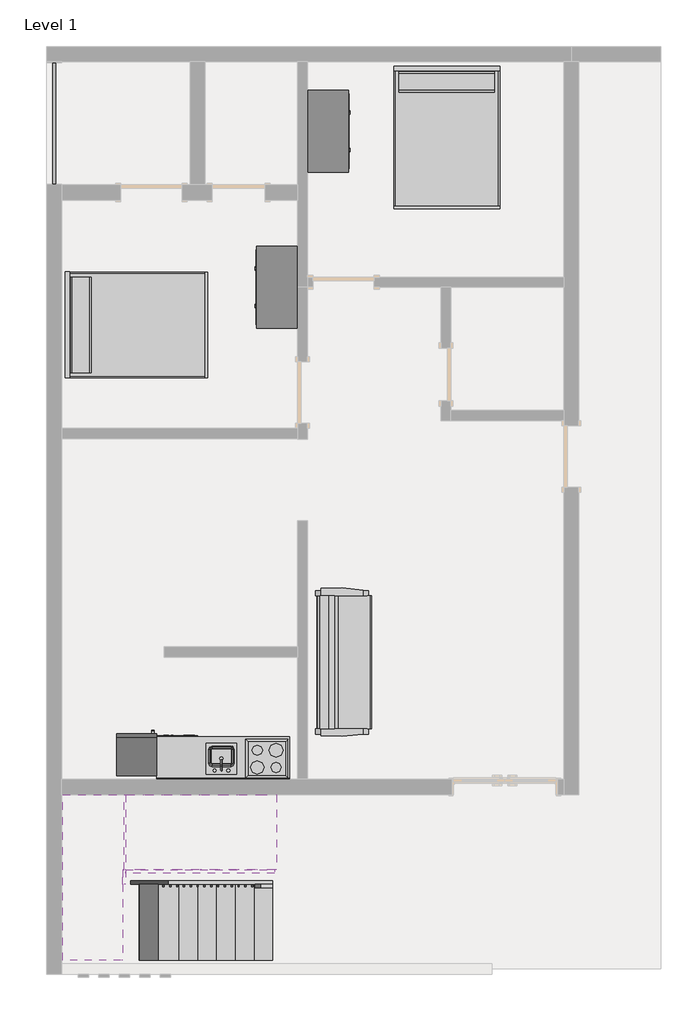
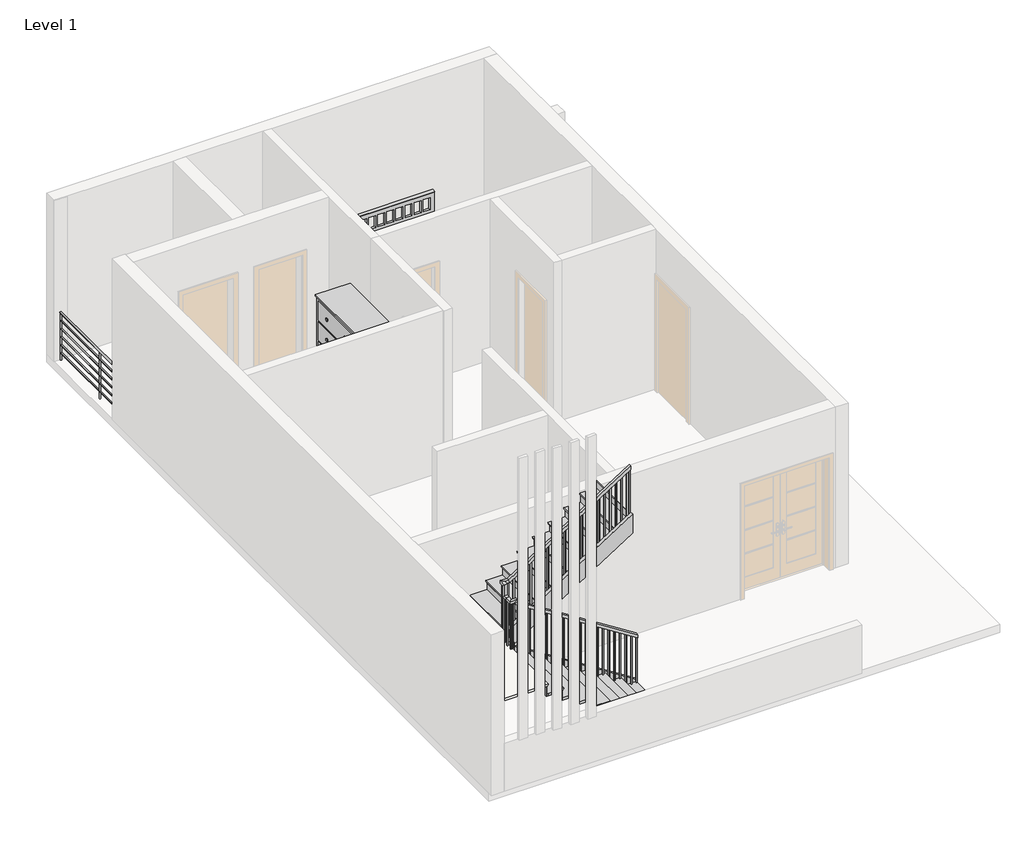
# One storey, part 2 of 2: 6 furniture elements, 4 proxies, 3 members, 2 railings, 2 stair flights, 1 flow terminal, 1 slab.
"""IFC4 building model written with IfcOpenShell, lengths in millimetres."""

from ifc_helpers import new_model, si_unit, point, frame, frame_2d, origin, origin_with_axes, place, context, project, spatial, polyline, circle_curve, trimmed, segment, composite_curve, outline, extrude, faceted_brep, transform, mapped, element, save
from components import proxy_a6faaae8, proxy_45b28599, kitchenette_medium_kitchenette_medium_844211aa, proxy_c523a7b7, flow_terminal_871c2e40, furniture_35c09872, furniture_c6510c7c, furniture_9fa109b2, furniture_aff9b2fb, non_monolithic_landing_c221236f, stair_flight_1352b5f3, stair_flight_ef2f52e6

model = new_model("IFC4")

# Units and contexts
model_context = context("Model", 3, world=origin())
ifc_project = project(units=[si_unit("LENGTHUNIT", "METRE", prefix="MILLI")], contexts=[model_context])

# Site, building, storey
site = spatial("IfcSite", under=ifc_project)
building = spatial("IfcBuilding", under=site)
storey = spatial("IfcBuildingStorey", under=building, Name="Level 1", Elevation=0.0)

# Proxies
placement = place(None, origin())
proxy_shape = proxy_a6faaae8(model_context)
element("IfcBuildingElementProxy", 1, Name="Cook Top-4 Unit2 : 22\" x 20\"", ObjectType="Cook Top-4 Unit2 : 22\" x 20\"", at=placement, inside=storey, context=model_context, shape_type="MappedRepresentation", body=[
    mapped(proxy_shape, transform((-8075.1683044, -841.1891189, 0.0), x_axis=(-1.0000000000000004, 0.0, 0.0), y_axis=(0.0, -1.0000000000000004, 0.0), z_axis=(0.0, 0.0, 1.0))),
])
proxy_2_shape = proxy_45b28599(model_context)
element("IfcBuildingElementProxy", 2, Name="Dishwasher : 24\" x 24\" x 34\"", ObjectType="Dishwasher : 24\" x 24\" x 34\"", at=placement, inside=storey, context=model_context, shape_type="MappedRepresentation", body=[
    mapped(proxy_2_shape, transform((-9026.3508359, -549.3395541, 0.0), x_axis=(-1.0000000000000004, 0.0, 0.0), y_axis=(0.0, -1.0000000000000004, 0.0), z_axis=(0.0, 0.0, 1.0))),
])
kitchenette_medium_kitchenette_medium_shape = kitchenette_medium_kitchenette_medium_844211aa(model_context)
element("IfcBuildingElementProxy", 3, Name="Kitchenette - Medium : Kitchenette - Medium", ObjectType="Kitchenette - Medium : Kitchenette - Medium", at=placement, inside=storey, context=model_context, shape_type="MappedRepresentation", body=[
    mapped(kitchenette_medium_kitchenette_medium_shape, transform((-8399.3305994, -1145.9891189, 0.0), x_axis=(-1.0000000000000004, 0.0, 0.0), y_axis=(0.0, -1.0000000000000004, 0.0), z_axis=(0.0, 0.0, 1.0))),
])
proxy_3_shape = proxy_c523a7b7(model_context)
element("IfcBuildingElementProxy", 4, Name="Refrigerator : 24\" x 25\" LH", ObjectType="Refrigerator : 24\" x 25\" LH", at=placement, inside=storey, context=model_context, shape_type="MappedRepresentation", body=[
    mapped(proxy_3_shape, transform((-10011.9183044, -795.5401474, 0.0), x_axis=(-1.0000000000000004, 0.0, 0.0), y_axis=(0.0, -1.0000000000000004, 0.0), z_axis=(0.0, 0.0, 1.0))),
])

# Flow terminal
flow_terminal_shape = flow_terminal_871c2e40(model_context)
element("IfcFlowTerminal", 5, ObjectType="Sink Kitchen-Island : 18\" x 18\"", at=placement, inside=storey, context=model_context, shape_type="MappedRepresentation", body=[
    mapped(flow_terminal_shape, transform((-8732.5790638, -838.8437178, -14.4), x_axis=(-1.0000000000000004, 0.0, 0.0), y_axis=(0.0, -1.0000000000000004, 0.0), z_axis=(0.0, 0.0, 1.0))),
])

# Furniture
furniture_shape = furniture_35c09872(model_context)
element("IfcFurniture", 6, ObjectType="Bed-Shaker : Queen 62\" x 83\"", at=placement, inside=storey, context=model_context, shape_type="MappedRepresentation", body=[
    mapped(furniture_shape, transform((-11059.6683044, 5629.4608811, 0.0), x_axis=(0.0, 1.0, 0.0), y_axis=(-1.0, 0.0, 0.0), z_axis=(0.0, 0.0, 1.0))),
])
element("IfcFurniture", 7, ObjectType="Bed-Shaker : Queen 62\" x 83\"", at=placement, inside=storey, context=model_context, shape_type="MappedRepresentation", body=[
    mapped(furniture_shape, transform((-5376.4183044, 9445.8108811, 0.0), x_axis=(1.0, 0.0, 0.0), y_axis=(0.0, 1.0, 0.0), z_axis=(0.0, 0.0, 1.0))),
])
furniture_2_shape = furniture_c6510c7c(model_context)
element("IfcFurniture", 8, ObjectType="Counter Top w Sink Hole : 24\" Depth", at=placement, inside=storey, context=model_context, shape_type="MappedRepresentation", body=[
    mapped(furniture_2_shape, transform((-8932.7305994, -1145.9891189, -14.4), x_axis=(-1.0000000000000004, 0.0, 0.0), y_axis=(0.0, -1.0000000000000004, 0.0), z_axis=(0.0, 0.0, 1.0))),
])
furniture_3_shape = furniture_9fa109b2(model_context)
element("IfcFurniture", 9, ObjectType="Dresser : 48\" x 72\" x 24\"", at=placement, inside=storey, context=model_context, shape_type="MappedRepresentation", body=[
    mapped(furniture_3_shape, transform((-7559.6053503, 5900.0176213, 0.0), x_axis=(0.0, -1.0000000000000004, 0.0), y_axis=(1.0000000000000004, 0.0, 0.0), z_axis=(0.0, 0.0, 1.0))),
])
element("IfcFurniture", 10, ObjectType="Dresser : 48\" x 72\" x 24\"", at=placement, inside=storey, context=model_context, shape_type="MappedRepresentation", body=[
    mapped(furniture_3_shape, transform((-7523.9312585, 8762.5041409, 0.0), x_axis=(0.0, 1.0000000000000009, 0.0), y_axis=(-1.0000000000000009, 0.0, 0.0), z_axis=(0.0, 0.0, 1.0))),
])
furniture_4_shape = furniture_aff9b2fb(model_context)
element("IfcFurniture", 11, ObjectType="Sofa-Pensi : 84\"", at=placement, inside=storey, context=model_context, shape_type="MappedRepresentation", body=[
    mapped(furniture_4_shape, transform((-6655.0584683, 315.3046311, 0.0), x_axis=(0.0, 1.0, 0.0), y_axis=(-1.0, 0.0, 0.0), z_axis=(0.0, 0.0, 1.0))),
])

# Members
element("IfcMember", 12, ObjectType="Stringer - 2\" Width", at=placement, inside=storey, context=model_context, shape_type="SweptSolid", body=[
    extrude(outline(polyline([(0.0, -7986.2683044), (215.0106437, -7986.2683044), (1605.083371, -10170.6683044), (1243.8010268, -10170.6683044), (0.0, -8216.1238337), (0.0, -7986.2683044)])), frame((0.0, -2706.1923176, 0.0), z_axis=(0.0, 1.0, 0.0), x_axis=(0.0, 0.0, 1.0)), (0.0, 0.0, 1.0), 50.8),
])
element("IfcMember", 13, ObjectType="Stringer - 2\" Width", at=placement, inside=storey, context=model_context, shape_type="SweptSolid", body=[
    extrude(outline(polyline([(1831.3742801, -10170.6683044), (1470.0919359, -10170.6683044), (2876.3282995, -7960.8683044), (3237.6106437, -7960.8683044), (1831.3742801, -10170.6683044)])), frame((0.0, -2542.9891189, 0.0), z_axis=(0.0, 1.0, 0.0), x_axis=(0.0, 0.0, 1.0)), (0.0, 0.0, 1.0), 50.8),
])
element("IfcMember", 14, ObjectType="Stringer - 2\" Width", at=placement, inside=storey, context=model_context, shape_type="SweptSolid", body=[
    extrude(outline(polyline([(-10170.6683044, -2706.1923176), (-10221.4683044, -2706.1923176), (-10221.4683044, -2492.1891189), (-10170.6683044, -2492.1891189), (-10170.6683044, -2706.1923176)])), frame((0.0, 0.0, 1371.6), z_axis=(0.0, 0.0, 1.0), x_axis=(1.0, 0.0, 0.0)), (0.0, 0.0, 1.0), 304.8),
])

# Railings
element("IfcRailing", 15, ObjectType="Handrail - Pipe", at=placement, inside=storey, context=model_context, shape_type="SweptSolid", body=[
    extrude(outline(composite_curve([segment(trimmed(circle_curve(frame_2d((895.35, -11237.4683044)), 19.05), [point((895.35, -11256.5183044))], [point((895.35, -11218.4183044))], False, "CARTESIAN"), True, "CONTINUOUS"), segment(trimmed(circle_curve(frame_2d((895.35, -11237.4683044)), 19.05), [point((895.35, -11218.4183044))], [point((895.35, -11256.5183044))], False, "CARTESIAN"), True, "CONTINUOUS")], self_intersect=False)), frame((0.0, 7705.9108811, 0.0), z_axis=(0.0, 1.0, 0.0), x_axis=(0.0, 0.0, 1.0)), (0.0, 0.0, 1.0), 1803.4),
    extrude(outline(composite_curve([segment(trimmed(circle_curve(frame_2d((749.3, -11237.4683044)), 12.7), [point((749.3, -11224.7683044))], [point((749.3, -11250.1683044))], False, "CARTESIAN"), True, "CONTINUOUS"), segment(trimmed(circle_curve(frame_2d((749.3, -11237.4683044)), 12.7), [point((749.3, -11250.1683044))], [point((749.3, -11224.7683044))], False, "CARTESIAN"), True, "CONTINUOUS")], self_intersect=False)), frame((0.0, 7705.9108811, 0.0), z_axis=(0.0, 1.0, 0.0), x_axis=(0.0, 0.0, 1.0)), (0.0, 0.0, 1.0), 1803.4),
    extrude(outline(composite_curve([segment(trimmed(circle_curve(frame_2d((596.9, -11237.4683044)), 12.7), [point((596.9, -11224.7683044))], [point((596.9, -11250.1683044))], False, "CARTESIAN"), True, "CONTINUOUS"), segment(trimmed(circle_curve(frame_2d((596.9, -11237.4683044)), 12.7), [point((596.9, -11250.1683044))], [point((596.9, -11224.7683044))], False, "CARTESIAN"), True, "CONTINUOUS")], self_intersect=False)), frame((0.0, 7705.9108811, 0.0), z_axis=(0.0, 1.0, 0.0), x_axis=(0.0, 0.0, 1.0)), (0.0, 0.0, 1.0), 1803.4),
    extrude(outline(composite_curve([segment(trimmed(circle_curve(frame_2d((444.5, -11237.4683044)), 12.7), [point((444.5, -11224.7683044))], [point((444.5, -11250.1683044))], False, "CARTESIAN"), True, "CONTINUOUS"), segment(trimmed(circle_curve(frame_2d((444.5, -11237.4683044)), 12.7), [point((444.5, -11250.1683044))], [point((444.5, -11224.7683044))], False, "CARTESIAN"), True, "CONTINUOUS")], self_intersect=False)), frame((0.0, 7705.9108811, 0.0), z_axis=(0.0, 1.0, 0.0), x_axis=(0.0, 0.0, 1.0)), (0.0, 0.0, 1.0), 1803.4),
    extrude(outline(composite_curve([segment(trimmed(circle_curve(frame_2d((292.1, -11237.4683044)), 12.7), [point((292.1, -11224.7683044))], [point((292.1, -11250.1683044))], False, "CARTESIAN"), True, "CONTINUOUS"), segment(trimmed(circle_curve(frame_2d((292.1, -11237.4683044)), 12.7), [point((292.1, -11250.1683044))], [point((292.1, -11224.7683044))], False, "CARTESIAN"), True, "CONTINUOUS")], self_intersect=False)), frame((0.0, 7705.9108811, 0.0), z_axis=(0.0, 1.0, 0.0), x_axis=(0.0, 0.0, 1.0)), (0.0, 0.0, 1.0), 1803.4),
    extrude(outline(composite_curve([segment(trimmed(circle_curve(frame_2d((139.7, -11237.4683044)), 12.7), [point((139.7, -11224.7683044))], [point((139.7, -11250.1683044))], False, "CARTESIAN"), True, "CONTINUOUS"), segment(trimmed(circle_curve(frame_2d((139.7, -11237.4683044)), 12.7), [point((139.7, -11250.1683044))], [point((139.7, -11224.7683044))], False, "CARTESIAN"), True, "CONTINUOUS")], self_intersect=False)), frame((0.0, 7705.9108811, 0.0), z_axis=(0.0, 1.0, 0.0), x_axis=(0.0, 0.0, 1.0)), (0.0, 0.0, 1.0), 1803.4),
    extrude(outline(composite_curve([segment(trimmed(circle_curve(frame_2d((-11237.4683044, 8290.1108811)), 12.7), [point((-11224.7683044, 8290.1108811))], [point((-11250.1683044, 8290.1108811))], False, "CARTESIAN"), True, "CONTINUOUS"), segment(trimmed(circle_curve(frame_2d((-11237.4683044, 8290.1108811)), 12.7), [point((-11250.1683044, 8290.1108811))], [point((-11224.7683044, 8290.1108811))], False, "CARTESIAN"), True, "CONTINUOUS")], self_intersect=False)), origin_with_axes(), (0.0, 0.0, 1.0), 876.3),
    extrude(outline(composite_curve([segment(trimmed(circle_curve(frame_2d((-11237.4683044, 7718.6108811)), 12.7), [point((-11224.7683044, 7718.6108811))], [point((-11250.1683044, 7718.6108811))], False, "CARTESIAN"), True, "CONTINUOUS"), segment(trimmed(circle_curve(frame_2d((-11237.4683044, 7718.6108811)), 12.7), [point((-11250.1683044, 7718.6108811))], [point((-11224.7683044, 7718.6108811))], False, "CARTESIAN"), True, "CONTINUOUS")], self_intersect=False)), origin_with_axes(), (0.0, 0.0, 1.0), 876.3),
    extrude(outline(composite_curve([segment(trimmed(circle_curve(frame_2d((-11237.4683044, 9496.6108811)), 12.7), [point((-11224.7683044, 9496.6108811))], [point((-11250.1683044, 9496.6108811))], False, "CARTESIAN"), True, "CONTINUOUS"), segment(trimmed(circle_curve(frame_2d((-11237.4683044, 9496.6108811)), 12.7), [point((-11250.1683044, 9496.6108811))], [point((-11224.7683044, 9496.6108811))], False, "CARTESIAN"), True, "CONTINUOUS")], self_intersect=False)), origin_with_axes(), (0.0, 0.0, 1.0), 876.3),
])
element("IfcRailing", 16, ObjectType="Handrail - Rectangular", at=placement, inside=storey, context=model_context, shape_type="SolidModel", body=[
    faceted_brep([(-7986.2683044, -2756.9923176, 1092.2), (-7986.2683044, -2756.9923176, 1031.986276), (-7986.2683044, -2706.1923176, 1031.986276), (-7986.2683044, -2706.1923176, 1092.2), (-10145.2683044, -2756.9923176, 2466.1090909), (-10196.0683044, -2756.9923176, 2438.2226396), (-10196.0683044, -2706.1923176, 2438.2226396), (-10145.2683044, -2706.1923176, 2466.1090909), (-10145.2683044, -2756.9923176, 2514.6), (-10196.0683044, -2756.9923176, 2463.8), (-10196.0683044, -2706.1923176, 2463.8), (-10145.2683044, -2706.1923176, 2514.6), (-10272.2683044, -2756.9923176, 2514.6), (-10272.2683044, -2756.9923176, 2463.8), (-10221.4683044, -2706.1923176, 2463.8), (-10221.4683044, -2706.1923176, 2514.6), (-10272.2683044, -2629.9923176, 2514.6), (-10272.2683044, -2629.9923176, 2463.8), (-10221.4683044, -2629.9923176, 2463.8), (-10221.4683044, -2629.9923176, 2514.6), (-10272.2683044, -2568.3891189, 2514.6), (-10272.2683044, -2517.5891189, 2463.8), (-10221.4683044, -2517.5891189, 2463.8), (-10221.4683044, -2568.3891189, 2514.6), (-10272.2683044, -2568.3891189, 2724.7272727), (-10272.2683044, -2517.5891189, 2673.9272727), (-10221.4683044, -2517.5891189, 2673.9272727), (-10221.4683044, -2568.3891189, 2724.7272727), (-7960.8683044, -2441.3891189, 4114.8), (-7960.8683044, -2492.1891189, 4114.8), (-7960.8683044, -2492.1891189, 4054.586276), (-7960.8683044, -2441.3891189, 4054.586276), (-10130.4753095, -2441.3891189, 2673.9272727), (-10145.2683044, -2441.3891189, 2724.7272727), (-10130.4753095, -2492.1891189, 2673.9272727), (-10145.2683044, -2492.1891189, 2724.7272727), (-10272.2683044, -2441.3891189, 2724.7272727), (-10272.2683044, -2441.3891189, 2673.9272727), (-10221.4683044, -2492.1891189, 2673.9272727), (-10221.4683044, -2492.1891189, 2724.7272727)], [[[0, 1, 2, 3]], [[1, 0, 4, 5]], [[2, 1, 5, 6]], [[3, 2, 6, 7]], [[0, 3, 7, 4]], [[5, 4, 8, 9]], [[6, 5, 9, 10]], [[7, 6, 10, 11]], [[4, 7, 11, 8]], [[9, 8, 12, 13]], [[10, 9, 13, 14]], [[11, 10, 14, 15]], [[8, 11, 15, 12]], [[13, 12, 16, 17]], [[14, 13, 17, 18]], [[15, 14, 18, 19]], [[12, 15, 19, 16]], [[17, 16, 20, 21]], [[18, 17, 21, 22]], [[19, 18, 22, 23]], [[16, 19, 23, 20]], [[21, 20, 24, 25]], [[22, 21, 25, 26]], [[23, 22, 26, 27]], [[20, 23, 27, 24]], [[28, 29, 30, 31]], [[32, 33, 28, 31]], [[34, 32, 31, 30]], [[35, 34, 30, 29]], [[33, 35, 29, 28]], [[25, 24, 36, 37]], [[26, 25, 37, 38]], [[27, 26, 38, 39]], [[24, 27, 39, 36]], [[37, 36, 33, 32]], [[38, 37, 32, 34]], [[39, 38, 34, 35]], [[36, 39, 35, 33]]]),
    extrude(outline(polyline([(4028.3203669, -8002.1433044), (4016.1976396, -8021.1933044), (3022.6, -8021.1933044), (3022.6, -8002.1433044), (4028.3203669, -8002.1433044)])), frame((0.0, -2476.3141189, 0.0), z_axis=(0.0, 1.0, 0.0), x_axis=(0.0, 0.0, 1.0)), (0.0, 0.0, 1.0), 19.05),
    extrude(outline(polyline([(3963.6658214, -8103.7433044), (3951.5430941, -8122.7933044), (3022.6, -8122.7933044), (3022.6, -8103.7433044), (3963.6658214, -8103.7433044)])), frame((0.0, -2476.3141189, 0.0), z_axis=(0.0, 1.0, 0.0), x_axis=(0.0, 0.0, 1.0)), (0.0, 0.0, 1.0), 19.05),
    extrude(outline(polyline([(3899.011276, -8205.3433044), (3886.8885487, -8224.3933044), (3022.6, -8224.3933044), (3022.6, -8205.3433044), (3899.011276, -8205.3433044)])), frame((0.0, -2476.3141189, 0.0), z_axis=(0.0, 1.0, 0.0), x_axis=(0.0, 0.0, 1.0)), (0.0, 0.0, 1.0), 19.05),
    extrude(outline(polyline([(3834.3567305, -8306.9433044), (3822.2340032, -8325.9933044), (2844.8, -8325.9933044), (2844.8, -8306.9433044), (3834.3567305, -8306.9433044)])), frame((0.0, -2476.3141189, 0.0), z_axis=(0.0, 1.0, 0.0), x_axis=(0.0, 0.0, 1.0)), (0.0, 0.0, 1.0), 19.05),
    extrude(outline(polyline([(3769.7021851, -8408.5433044), (3757.5794578, -8427.5933044), (2844.8, -8427.5933044), (2844.8, -8408.5433044), (3769.7021851, -8408.5433044)])), frame((0.0, -2476.3141189, 0.0), z_axis=(0.0, 1.0, 0.0), x_axis=(0.0, 0.0, 1.0)), (0.0, 0.0, 1.0), 19.05),
    extrude(outline(polyline([(3705.0476396, -8510.1433044), (3692.9249123, -8529.1933044), (2844.8, -8529.1933044), (2844.8, -8510.1433044), (3705.0476396, -8510.1433044)])), frame((0.0, -2476.3141189, 0.0), z_axis=(0.0, 1.0, 0.0), x_axis=(0.0, 0.0, 1.0)), (0.0, 0.0, 1.0), 19.05),
    extrude(outline(polyline([(3640.3930941, -8611.7433044), (3628.2703669, -8630.7933044), (2667.0, -8630.7933044), (2667.0, -8611.7433044), (3640.3930941, -8611.7433044)])), frame((0.0, -2476.3141189, 0.0), z_axis=(0.0, 1.0, 0.0), x_axis=(0.0, 0.0, 1.0)), (0.0, 0.0, 1.0), 19.05),
    extrude(outline(polyline([(3575.7385487, -8713.3433044), (3563.6158214, -8732.3933044), (2667.0, -8732.3933044), (2667.0, -8713.3433044), (3575.7385487, -8713.3433044)])), frame((0.0, -2476.3141189, 0.0), z_axis=(0.0, 1.0, 0.0), x_axis=(0.0, 0.0, 1.0)), (0.0, 0.0, 1.0), 19.05),
    extrude(outline(polyline([(3511.0840032, -8814.9433044), (3498.961276, -8833.9933044), (2489.2, -8833.9933044), (2489.2, -8814.9433044), (3511.0840032, -8814.9433044)])), frame((0.0, -2476.3141189, 0.0), z_axis=(0.0, 1.0, 0.0), x_axis=(0.0, 0.0, 1.0)), (0.0, 0.0, 1.0), 19.05),
    extrude(outline(polyline([(3446.4294578, -8916.5433044), (3434.3067305, -8935.5933044), (2489.2, -8935.5933044), (2489.2, -8916.5433044), (3446.4294578, -8916.5433044)])), frame((0.0, -2476.3141189, 0.0), z_axis=(0.0, 1.0, 0.0), x_axis=(0.0, 0.0, 1.0)), (0.0, 0.0, 1.0), 19.05),
    extrude(outline(polyline([(3381.7749123, -9018.1433044), (3369.6521851, -9037.1933044), (2489.2, -9037.1933044), (2489.2, -9018.1433044), (3381.7749123, -9018.1433044)])), frame((0.0, -2476.3141189, 0.0), z_axis=(0.0, 1.0, 0.0), x_axis=(0.0, 0.0, 1.0)), (0.0, 0.0, 1.0), 19.05),
    extrude(outline(polyline([(3317.1203669, -9119.7433044), (3304.9976396, -9138.7933044), (2311.4, -9138.7933044), (2311.4, -9119.7433044), (3317.1203669, -9119.7433044)])), frame((0.0, -2476.3141189, 0.0), z_axis=(0.0, 1.0, 0.0), x_axis=(0.0, 0.0, 1.0)), (0.0, 0.0, 1.0), 19.05),
    extrude(outline(polyline([(3252.4658214, -9221.3433044), (3240.3430941, -9240.3933044), (2311.4, -9240.3933044), (2311.4, -9221.3433044), (3252.4658214, -9221.3433044)])), frame((0.0, -2476.3141189, 0.0), z_axis=(0.0, 1.0, 0.0), x_axis=(0.0, 0.0, 1.0)), (0.0, 0.0, 1.0), 19.05),
    extrude(outline(polyline([(3187.811276, -9322.9433044), (3175.6885487, -9341.9933044), (2311.4, -9341.9933044), (2311.4, -9322.9433044), (3187.811276, -9322.9433044)])), frame((0.0, -2476.3141189, 0.0), z_axis=(0.0, 1.0, 0.0), x_axis=(0.0, 0.0, 1.0)), (0.0, 0.0, 1.0), 19.05),
    extrude(outline(polyline([(3123.1567305, -9424.5433044), (3111.0340032, -9443.5933044), (2133.6, -9443.5933044), (2133.6, -9424.5433044), (3123.1567305, -9424.5433044)])), frame((0.0, -2476.3141189, 0.0), z_axis=(0.0, 1.0, 0.0), x_axis=(0.0, 0.0, 1.0)), (0.0, 0.0, 1.0), 19.05),
    extrude(outline(polyline([(3058.5021851, -9526.1433044), (3046.3794578, -9545.1933044), (2133.6, -9545.1933044), (2133.6, -9526.1433044), (3058.5021851, -9526.1433044)])), frame((0.0, -2476.3141189, 0.0), z_axis=(0.0, 1.0, 0.0), x_axis=(0.0, 0.0, 1.0)), (0.0, 0.0, 1.0), 19.05),
    extrude(outline(polyline([(2993.8476396, -9627.7433044), (2981.7249123, -9646.7933044), (2133.6, -9646.7933044), (2133.6, -9627.7433044), (2993.8476396, -9627.7433044)])), frame((0.0, -2476.3141189, 0.0), z_axis=(0.0, 1.0, 0.0), x_axis=(0.0, 0.0, 1.0)), (0.0, 0.0, 1.0), 19.05),
    extrude(outline(polyline([(2929.1930941, -9729.3433044), (2917.0703669, -9748.3933044), (1955.8, -9748.3933044), (1955.8, -9729.3433044), (2929.1930941, -9729.3433044)])), frame((0.0, -2476.3141189, 0.0), z_axis=(0.0, 1.0, 0.0), x_axis=(0.0, 0.0, 1.0)), (0.0, 0.0, 1.0), 19.05),
    extrude(outline(polyline([(2864.5385487, -9830.9433044), (2852.4158214, -9849.9933044), (1955.8, -9849.9933044), (1955.8, -9830.9433044), (2864.5385487, -9830.9433044)])), frame((0.0, -2476.3141189, 0.0), z_axis=(0.0, 1.0, 0.0), x_axis=(0.0, 0.0, 1.0)), (0.0, 0.0, 1.0), 19.05),
    extrude(outline(polyline([(2799.8840032, -9932.5433044), (2787.761276, -9951.5933044), (1778.0, -9951.5933044), (1778.0, -9932.5433044), (2799.8840032, -9932.5433044)])), frame((0.0, -2476.3141189, 0.0), z_axis=(0.0, 1.0, 0.0), x_axis=(0.0, 0.0, 1.0)), (0.0, 0.0, 1.0), 19.05),
    extrude(outline(polyline([(2735.2294578, -10034.1433044), (2723.1067305, -10053.1933044), (1778.0, -10053.1933044), (1778.0, -10034.1433044), (2735.2294578, -10034.1433044)])), frame((0.0, -2476.3141189, 0.0), z_axis=(0.0, 1.0, 0.0), x_axis=(0.0, 0.0, 1.0)), (0.0, 0.0, 1.0), 19.05),
    extrude(outline(polyline([(-10154.7933044, -2476.3141189), (-10154.7933044, -2457.2641189), (-10135.7433044, -2457.2641189), (-10135.7433044, -2476.3141189), (-10154.7933044, -2476.3141189)])), frame((0.0, 0.0, 1778.0), z_axis=(0.0, 0.0, 1.0), x_axis=(1.0, 0.0, 0.0)), (0.0, 0.0, 1.0), 895.9272727),
    extrude(outline(polyline([(-10237.3433044, -2537.9173176), (-10256.3933044, -2537.9173176), (-10256.3933044, -2518.8673176), (-10237.3433044, -2518.8673176), (-10237.3433044, -2537.9173176)])), frame((0.0, 0.0, 1600.2), z_axis=(0.0, 0.0, 1.0), x_axis=(1.0, 0.0, 0.0)), (0.0, 0.0, 1.0), 863.6),
    extrude(outline(polyline([(-10237.3433044, -2639.5173176), (-10256.3933044, -2639.5173176), (-10256.3933044, -2620.4673176), (-10237.3433044, -2620.4673176), (-10237.3433044, -2639.5173176)])), frame((0.0, 0.0, 1600.2), z_axis=(0.0, 0.0, 1.0), x_axis=(1.0, 0.0, 0.0)), (0.0, 0.0, 1.0), 863.6),
    extrude(outline(polyline([(2383.6703669, -10110.3433044), (2395.7930941, -10129.3933044), (1422.4, -10129.3933044), (1422.4, -10110.3433044), (2383.6703669, -10110.3433044)])), frame((0.0, -2741.1173176, 0.0), z_axis=(0.0, 1.0, 0.0), x_axis=(0.0, 0.0, 1.0)), (0.0, 0.0, 1.0), 19.05),
    extrude(outline(polyline([(2319.0158214, -10008.7433044), (2331.1385487, -10027.7933044), (1422.4, -10027.7933044), (1422.4, -10008.7433044), (2319.0158214, -10008.7433044)])), frame((0.0, -2741.1173176, 0.0), z_axis=(0.0, 1.0, 0.0), x_axis=(0.0, 0.0, 1.0)), (0.0, 0.0, 1.0), 19.05),
    extrude(outline(polyline([(2254.361276, -9907.1433044), (2266.4840032, -9926.1933044), (1244.6, -9926.1933044), (1244.6, -9907.1433044), (2254.361276, -9907.1433044)])), frame((0.0, -2741.1173176, 0.0), z_axis=(0.0, 1.0, 0.0), x_axis=(0.0, 0.0, 1.0)), (0.0, 0.0, 1.0), 19.05),
    extrude(outline(polyline([(2189.7067305, -9805.5433044), (2201.8294578, -9824.5933044), (1244.6, -9824.5933044), (1244.6, -9805.5433044), (2189.7067305, -9805.5433044)])), frame((0.0, -2741.1173176, 0.0), z_axis=(0.0, 1.0, 0.0), x_axis=(0.0, 0.0, 1.0)), (0.0, 0.0, 1.0), 19.05),
    extrude(outline(polyline([(2125.0521851, -9703.9433044), (2137.1749123, -9722.9933044), (1244.6, -9722.9933044), (1244.6, -9703.9433044), (2125.0521851, -9703.9433044)])), frame((0.0, -2741.1173176, 0.0), z_axis=(0.0, 1.0, 0.0), x_axis=(0.0, 0.0, 1.0)), (0.0, 0.0, 1.0), 19.05),
    extrude(outline(polyline([(2060.3976396, -9602.3433044), (2072.5203669, -9621.3933044), (1066.8, -9621.3933044), (1066.8, -9602.3433044), (2060.3976396, -9602.3433044)])), frame((0.0, -2741.1173176, 0.0), z_axis=(0.0, 1.0, 0.0), x_axis=(0.0, 0.0, 1.0)), (0.0, 0.0, 1.0), 19.05),
    extrude(outline(polyline([(1995.7430941, -9500.7433044), (2007.8658214, -9519.7933044), (1066.8, -9519.7933044), (1066.8, -9500.7433044), (1995.7430941, -9500.7433044)])), frame((0.0, -2741.1173176, 0.0), z_axis=(0.0, 1.0, 0.0), x_axis=(0.0, 0.0, 1.0)), (0.0, 0.0, 1.0), 19.05),
    extrude(outline(polyline([(1931.0885487, -9399.1433044), (1943.211276, -9418.1933044), (1066.8, -9418.1933044), (1066.8, -9399.1433044), (1931.0885487, -9399.1433044)])), frame((0.0, -2741.1173176, 0.0), z_axis=(0.0, 1.0, 0.0), x_axis=(0.0, 0.0, 1.0)), (0.0, 0.0, 1.0), 19.05),
    extrude(outline(polyline([(1866.4340032, -9297.5433044), (1878.5567305, -9316.5933044), (889.0, -9316.5933044), (889.0, -9297.5433044), (1866.4340032, -9297.5433044)])), frame((0.0, -2741.1173176, 0.0), z_axis=(0.0, 1.0, 0.0), x_axis=(0.0, 0.0, 1.0)), (0.0, 0.0, 1.0), 19.05),
    extrude(outline(polyline([(1801.7794578, -9195.9433044), (1813.9021851, -9214.9933044), (889.0, -9214.9933044), (889.0, -9195.9433044), (1801.7794578, -9195.9433044)])), frame((0.0, -2741.1173176, 0.0), z_axis=(0.0, 1.0, 0.0), x_axis=(0.0, 0.0, 1.0)), (0.0, 0.0, 1.0), 19.05),
    extrude(outline(polyline([(1737.1249123, -9094.3433044), (1749.2476396, -9113.3933044), (889.0, -9113.3933044), (889.0, -9094.3433044), (1737.1249123, -9094.3433044)])), frame((0.0, -2741.1173176, 0.0), z_axis=(0.0, 1.0, 0.0), x_axis=(0.0, 0.0, 1.0)), (0.0, 0.0, 1.0), 19.05),
    extrude(outline(polyline([(1672.4703669, -8992.7433044), (1684.5930941, -9011.7933044), (711.2, -9011.7933044), (711.2, -8992.7433044), (1672.4703669, -8992.7433044)])), frame((0.0, -2741.1173176, 0.0), z_axis=(0.0, 1.0, 0.0), x_axis=(0.0, 0.0, 1.0)), (0.0, 0.0, 1.0), 19.05),
    extrude(outline(polyline([(1607.8158214, -8891.1433044), (1619.9385487, -8910.1933044), (711.2, -8910.1933044), (711.2, -8891.1433044), (1607.8158214, -8891.1433044)])), frame((0.0, -2741.1173176, 0.0), z_axis=(0.0, 1.0, 0.0), x_axis=(0.0, 0.0, 1.0)), (0.0, 0.0, 1.0), 19.05),
    extrude(outline(polyline([(1543.161276, -8789.5433044), (1555.2840032, -8808.5933044), (533.4, -8808.5933044), (533.4, -8789.5433044), (1543.161276, -8789.5433044)])), frame((0.0, -2741.1173176, 0.0), z_axis=(0.0, 1.0, 0.0), x_axis=(0.0, 0.0, 1.0)), (0.0, 0.0, 1.0), 19.05),
    extrude(outline(polyline([(1478.5067305, -8687.9433044), (1490.6294578, -8706.9933044), (533.4, -8706.9933044), (533.4, -8687.9433044), (1478.5067305, -8687.9433044)])), frame((0.0, -2741.1173176, 0.0), z_axis=(0.0, 1.0, 0.0), x_axis=(0.0, 0.0, 1.0)), (0.0, 0.0, 1.0), 19.05),
    extrude(outline(polyline([(1413.8521851, -8586.3433044), (1425.9749123, -8605.3933044), (533.4, -8605.3933044), (533.4, -8586.3433044), (1413.8521851, -8586.3433044)])), frame((0.0, -2741.1173176, 0.0), z_axis=(0.0, 1.0, 0.0), x_axis=(0.0, 0.0, 1.0)), (0.0, 0.0, 1.0), 19.05),
    extrude(outline(polyline([(1349.1976396, -8484.7433044), (1361.3203669, -8503.7933044), (355.6, -8503.7933044), (355.6, -8484.7433044), (1349.1976396, -8484.7433044)])), frame((0.0, -2741.1173176, 0.0), z_axis=(0.0, 1.0, 0.0), x_axis=(0.0, 0.0, 1.0)), (0.0, 0.0, 1.0), 19.05),
    extrude(outline(polyline([(1284.5430941, -8383.1433044), (1296.6658214, -8402.1933044), (355.6, -8402.1933044), (355.6, -8383.1433044), (1284.5430941, -8383.1433044)])), frame((0.0, -2741.1173176, 0.0), z_axis=(0.0, 1.0, 0.0), x_axis=(0.0, 0.0, 1.0)), (0.0, 0.0, 1.0), 19.05),
    extrude(outline(polyline([(1219.8885487, -8281.5433044), (1232.011276, -8300.5933044), (355.6, -8300.5933044), (355.6, -8281.5433044), (1219.8885487, -8281.5433044)])), frame((0.0, -2741.1173176, 0.0), z_axis=(0.0, 1.0, 0.0), x_axis=(0.0, 0.0, 1.0)), (0.0, 0.0, 1.0), 19.05),
    extrude(outline(polyline([(1155.2340032, -8179.9433044), (1167.3567305, -8198.9933044), (177.8, -8198.9933044), (177.8, -8179.9433044), (1155.2340032, -8179.9433044)])), frame((0.0, -2741.1173176, 0.0), z_axis=(0.0, 1.0, 0.0), x_axis=(0.0, 0.0, 1.0)), (0.0, 0.0, 1.0), 19.05),
    extrude(outline(polyline([(1090.5794578, -8078.3433044), (1102.7021851, -8097.3933044), (177.8, -8097.3933044), (177.8, -8078.3433044), (1090.5794578, -8078.3433044)])), frame((0.0, -2741.1173176, 0.0), z_axis=(0.0, 1.0, 0.0), x_axis=(0.0, 0.0, 1.0)), (0.0, 0.0, 1.0), 19.05),
    extrude(outline(polyline([(-10256.3933044, -2476.3141189), (-10256.3933044, -2457.2641189), (-10237.3433044, -2457.2641189), (-10237.3433044, -2476.3141189), (-10256.3933044, -2476.3141189)])), frame((0.0, 0.0, 1600.2), z_axis=(0.0, 0.0, 1.0), x_axis=(1.0, 0.0, 0.0)), (0.0, 0.0, 1.0), 1073.7272727),
    extrude(outline(polyline([(-10237.3433044, -2722.0673176), (-10237.3433044, -2741.1173176), (-10256.3933044, -2741.1173176), (-10256.3933044, -2722.0673176), (-10237.3433044, -2722.0673176)])), frame((0.0, 0.0, 1600.2), z_axis=(0.0, 0.0, 1.0), x_axis=(1.0, 0.0, 0.0)), (0.0, 0.0, 1.0), 863.6),
    extrude(outline(polyline([(-10211.9433044, -2722.0673176), (-10211.9433044, -2741.1173176), (-10230.9933044, -2741.1173176), (-10230.9933044, -2722.0673176), (-10211.9433044, -2722.0673176)])), frame((0.0, 0.0, 1600.2), z_axis=(0.0, 0.0, 1.0), x_axis=(1.0, 0.0, 0.0)), (0.0, 0.0, 1.0), 863.6),
    extrude(outline(polyline([(4054.586276, -7960.8683044), (4042.4635487, -7979.9183044), (3022.6, -7979.9183044), (3022.6, -7960.8683044), (4054.586276, -7960.8683044)])), frame((0.0, -2476.3141189, 0.0), z_axis=(0.0, 1.0, 0.0), x_axis=(0.0, 0.0, 1.0)), (0.0, 0.0, 1.0), 19.05),
    extrude(outline(polyline([(1031.986276, -7986.2683044), (1044.1090032, -8005.3183044), (177.8, -8005.3183044), (177.8, -7986.2683044), (1031.986276, -7986.2683044)])), frame((0.0, -2741.1173176, 0.0), z_axis=(0.0, 1.0, 0.0), x_axis=(0.0, 0.0, 1.0)), (0.0, 0.0, 1.0), 19.05),
])

# Slab
non_monolithic_landing_shape = non_monolithic_landing_c221236f(model_context)
element("IfcSlab", 17, ObjectType="Non-Monolithic Landing", at=placement, inside=storey, context=model_context, shape_type="MappedRepresentation", body=[
    mapped(non_monolithic_landing_shape, transform((0.0, 0.0, 0.0), x_axis=(1.0, 0.0, 0.0), y_axis=(0.0, 1.0, 0.0), z_axis=(0.0, 0.0, 1.0))),
])

# Stair flights
stair_flight_shape = stair_flight_1352b5f3(model_context)
element("IfcStairFlight", 18, ObjectType="2\" Tread 1\" Nosing 1/4\" Riser", at=placement, inside=storey, context=model_context, shape_type="MappedRepresentation", body=[
    mapped(stair_flight_shape, transform((0.0, 0.0, 0.0), x_axis=(1.0, 0.0, 0.0), y_axis=(0.0, 1.0, 0.0), z_axis=(0.0, 0.0, 1.0))),
])
stair_flight_2_shape = stair_flight_ef2f52e6(model_context)
element("IfcStairFlight", 19, ObjectType="2\" Tread 1\" Nosing 1/4\" Riser", at=placement, inside=storey, context=model_context, shape_type="MappedRepresentation", body=[
    mapped(stair_flight_2_shape, transform((0.0, 0.0, 0.0), x_axis=(1.0, 0.0, 0.0), y_axis=(0.0, 1.0, 0.0), z_axis=(0.0, 0.0, 1.0))),
])

save(model, "model.ifc")

# Revit data of these elements
# Type "Cook Top-4 Unit2 : 22\" x 20\""
#   Depth = 1' - 8"
#   Width = 1' - 10"
#   Burner Material = Steel, Chrome Plated
#   Cooktop Material = Steel, Polished
#   Default Elevation = 0
#   Assembly Code = ""
# Type "Dishwasher : 24\" x 24\" x 34\""
#   Label = "DW"
#   Assembly Code = "E1090400"
#   Depth = 2' - 0"
#   Height = 2' - 10"
#   Width = 2' - 0"
#   Dishwasher Material = Steel, Paint Finish, Ivory, Glossy
#   Panel Face Material = Plastic, Opaque Black
#   Default Elevation = 0
# Type "Kitchenette - Medium : Kitchenette - Medium"
#   Assembly Code = "E1090400"
#   Counter Length = 6' - 6"
#   Cabinet Width = 4' - 6"
#   Cabinet Height = 2' - 10 1/2"
#   Cabinet Depth = 2' - 0"
#   Toe Depth = 0' - 3"
#   Toe Height = 0' - 3 1/2"
#   Cabinet Material = Cabinets
#   Door/Drawer Material = Cabinets
#   Handle Material = Cabinets - Handles
#   Default Elevation = 0
# Type "Refrigerator : 24\" x 25\" LH"
#   Label = "REF."
#   Assembly Code = "E1090400"
#   Depth = 2' - 0 3/4"
#   Handle = 0' - 1 1/2"
#   Height = 5' - 3 1/2"
#   Rear Clearance = 0' - 2"
#   Top Door Height = 1' - 8"
#   Width = 1' - 11 1/2"
#   Material = Steel, Paint Finish, Ivory, Glossy
#   Default Elevation = 0
# Type "Sink Kitchen-Island : 18\" x 18\""
#   Assembly Code = "D2010410"
#   Counter Height = 3' - 0"
#   Depth = 1' - 6"
#   Width = 1' - 6"
#   Faucet Material = Steel, Polished
#   Sink Material = Steel, Polished
#   Default Elevation = 0
# Type "Bed-Shaker : Queen 62\" x 83\""
#   Assembly Code = "E2020200"
#   Length = 6' - 11"
#   Width = 5' - 2"
#   Frame Material = Birch
#   Mattress Material = Linen, White
#   Default Elevation = 0
# Type "Counter Top w Sink Hole : 24\" Depth"
#   Assembly Code = "C1030400"
#   Counter Thickness = 0' - 1 1/2"
#   Depth = 2' - 1"
#   Height = 3' - 0"
#   Length [instance default] = 8' - 0"
#   Sink Location [instance default] = 2' - 0"
#   Sink Location To Wall [instance default] = 0' - 6"
#   Sink Opening Depth [instance default] = 1' - 3"
#   Sink Opening Width [instance default] = 2' - 3"
#   Counter Top Material = none
#   Default Elevation = 0
# Type "Dresser : 48\" x 72\" x 24\""
#   Assembly Code = "E2020200"
#   Depth = 2' - 0"
#   Height = 6' - 0"
#   Width = 4' - 0"
#   Dresser Material = Laminate - Ivory, Glossy
#   Drawer Material = Laminate, Ivory, Matte
#   Knob Material = Cherry
#   Default Elevation = 0
# Type "Sofa-Pensi : 84\""
#   Assembly Code = "E2020200"
#   Length = 7' - 0"
#   Frame Material = Cherry
#   Seat Material = Linen, Beige
#   Feet Material = Steel, Chrome Plated
#   Default Elevation = 0
# Type "Handrail - Pipe"
#   Assembly Code = "C2010400"
#   built-in parameter 1008612 = 0.0416667 (stored number, unit not read)
#   built-in parameter 1008611 = 0.0833333 (stored number, unit not read)
#   built-in parameter 1008609 = 4 (stored number, unit not read)
#   built-in parameter 1008604 = 0.166667 (stored number, unit not read)
#   built-in parameter 1008603 = 0.166667 (stored number, unit not read)
#   Railing Height = 3' - 0"
#   built-in parameter 1008630 = 2
#   built-in parameter 1008610 = 1
#   built-in parameter 1008605 = 1
#   built-in parameter 1008618 = Baluster - Round : 1"
# Type "Handrail - Rectangular"
#   Assembly Code = "C2010400"
#   built-in parameter 1008612 = 0.0416667 (stored number, unit not read)
#   built-in parameter 1008611 = 0.0416667 (stored number, unit not read)
#   built-in parameter 1008609 = 0.333333 (stored number, unit not read)
#   built-in parameter 1008604 = 0.166667 (stored number, unit not read)
#   built-in parameter 1008603 = 0.166667 (stored number, unit not read)
#   Railing Height = 3' - 0"
#   built-in parameter 1008630 = 2
#   built-in parameter 1008610 = 2
#   built-in parameter 1008618 = Baluster - Square : 3/4"
# Element 1 (IfcBuildingElementProxy, "Cook Top-4 Unit2 : 22\" x 20\"")
#   Phase Created = New Construction
#   Materials on its faces: "Steel, Chrome Plated", "Steel, Polished"
# Element 2 (IfcBuildingElementProxy, "Dishwasher : 24\" x 24\" x 34\"")
#   Phase Created = New Construction
#   Materials on its faces: "Steel, Paint Finish, Ivory, Glossy", "Plastic, Opaque Black"
# Element 3 (IfcBuildingElementProxy, "Kitchenette - Medium : Kitchenette - Medium")
#   Phase Created = New Construction
#   Materials on its faces: "Cabinets", "Cabinets - Handles"
# Element 4 (IfcBuildingElementProxy, "Refrigerator : 24\" x 25\" LH")
#   Phase Created = New Construction
#   Materials on its faces: "Steel, Paint Finish, Ivory, Glossy", "Steel, Chrome Plated"
# Element 5 (IfcFlowTerminal, "Sink Kitchen-Island : 18\" x 18\"")
#   Mark = "3"
#   Phase Created = New Construction
#   Materials on its faces: "Steel, Polished"
# Elements 6, 7 (IfcFurniture, "Bed-Shaker : Queen 62\" x 83\"")
#   Phase Created = New Construction
#   Materials on its faces: "Birch", "Linen, White"
# Element 8 (IfcFurniture, "Counter Top w Sink Hole : 24\" Depth")
#   Sink Opening Depth = 1' - 2"
#   Sink Location To Wall = 0' - 6"
#   Length = 6' - 6"
#   Sink Location = 3' - 4"
#   Sink Opening Width = 1' - 4"
#   Phase Created = New Construction
#   Materials on its faces: "Counter Top"
# Elements 9, 10 (IfcFurniture, "Dresser : 48\" x 72\" x 24\"")
#   Phase Created = New Construction
#   Materials on its faces: "Laminate, Ivory, Matte", "Cherry", "Laminate - Ivory, Glossy"
# Element 11 (IfcFurniture, "Sofa-Pensi : 84\"")
#   Phase Created = New Construction
#   Materials on its faces: "Cherry", "Linen, Beige", "Steel, Chrome Plated"
# Elements 12, 13, 14 (IfcMember, "Stringer - 2\" Width")
#   Phase Created = New Construction
# Element 15 (IfcRailing, "Handrail - Pipe")
#   Phase Created = New Construction
# Element 16 (IfcRailing, "Handrail - Rectangular")
#   Phase Created = New Construction
# Element 17 (IfcSlab, "Non-Monolithic Landing")
#   Phase Created = New Construction
# Elements 18, 19 (IfcStairFlight, "2\" Tread 1\" Nosing 1/4\" Riser")
#   Phase Created = New Construction
# Materials
#   "Steel, Chrome Plated": class "Metal", colour RGB 17 17 17, transparency 0, Description = "Chromiuim plated steel", Cost = 0
#   "Steel, Polished": class "Metal", colour RGB 57 57 57, transparency 0, Description = "Polished steel", Cost = 0
#   "Steel, Paint Finish, Ivory, Glossy": class "Metal", colour RGB 247 247 239, transparency 0, Description = "Steel, paint finish, ivory, glossy", Cost = 0
#   "Plastic, Opaque Black": class "Plastic", colour RGB 0 0 0, transparency 0.7, Description = "Plastic, generic, opaque black", Cost = 0
#   "Cabinets": colour RGB 249 249 249, transparency 0
#   "Cabinets - Handles": class "Metal", colour RGB 57 57 57, transparency 0
#   "Birch": class "Wood", colour RGB 224 178 126, transparency 0, Description = "Betula Alleghaniensis", Cost = 0
#   "Linen, White": class "Textile", colour RGB 247 247 239, transparency 0, Description = "Linen, white", Cost = 0
#   "Laminate - Ivory, Glossy": colour RGB 247 247 239, transparency 0
#   "Laminate, Ivory, Matte": class "Plastic", colour RGB 247 247 239, transparency 0, Description = "Plastic Laminate - Ivory, Matte", Cost = 0
#   "Cherry": class "Wood", colour RGB 226 177 128, transparency 0, Description = "Prunus Serotina", Cost = 0
#   "Linen, Beige": class "Textile", colour RGB 249 239 230, transparency 0, Description = "Linen, beige", Cost = 0
#   "Counter Top": class "Wood", colour RGB 226 177 128, transparency 0
